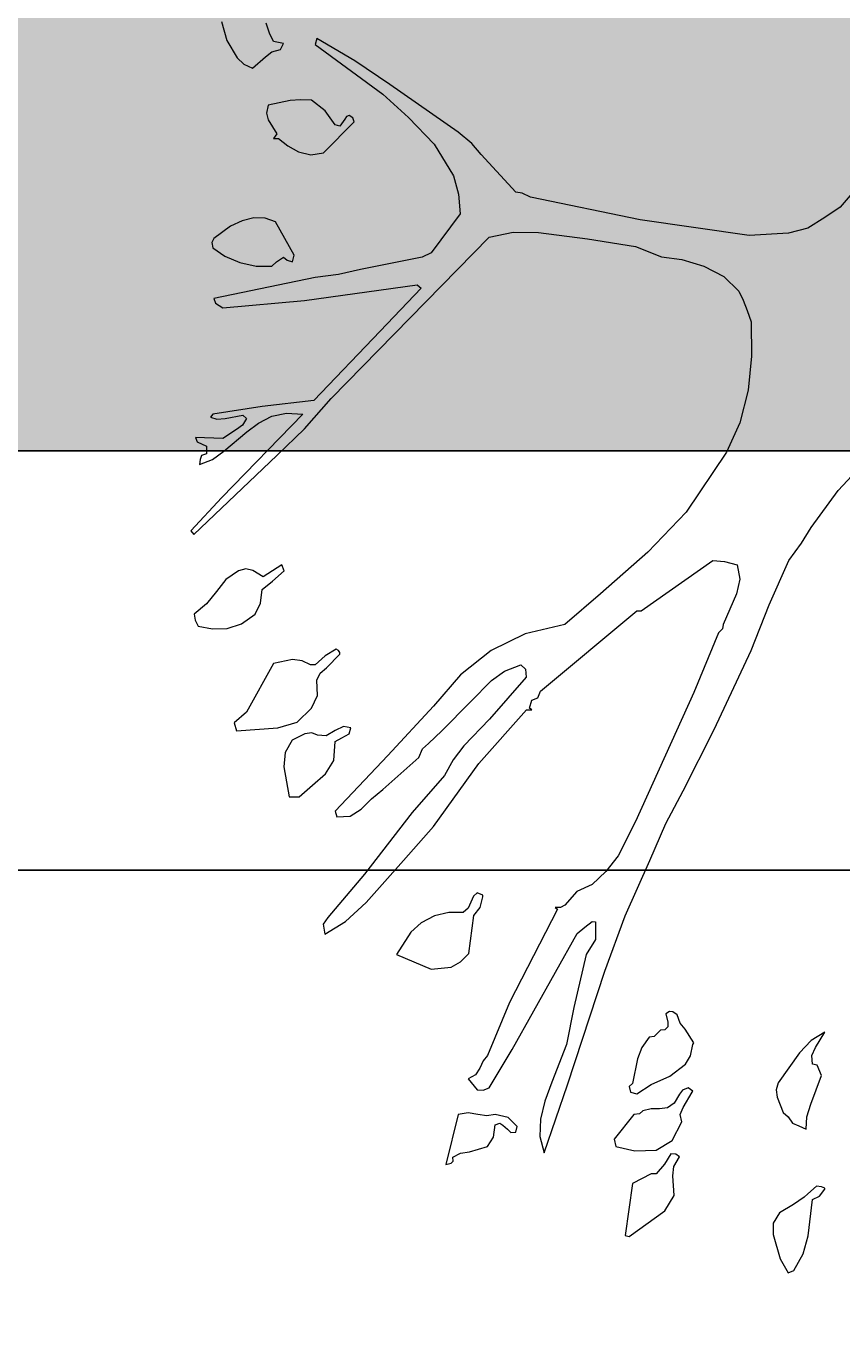
# Model space of a CAD drawing. Units: inches. Extents: x 84 to 1044, y -280 to 906.
# Tile 6 of 105: x 481 to 498, y -132 to -104. Entities that reach past the tile are written whole.
import ezdxf

# ---------------------------------------------------------------- set-up
doc = ezdxf.new("R2010")
doc.units = ezdxf.units.IN
for name, color, linetype, lineweight in [('A-ANNO-DIMS', 2, 'Continuous', 18), ('C-PROP', 7, 'Continuous', 25), ('L-PLNT', 114, 'Continuous', 15)]:
    doc.layers.add(name, color=color, linetype=linetype, lineweight=lineweight)
doc.layers.add('L-PLNT-PATT', color=9, linetype='Continuous', lineweight=9, true_color=0xafd9aa)
doc.styles.get("Standard").update_dxf_attribs({"font": 'arial.ttf'})
doc.dimstyles.get("Standard").update_dxf_attribs({"dimtxt": 0.18, "dimasz": 0.18, "dimexe": 0.18, "dimexo": 0.0625, "dimgap": 0.09, "dimtad": 0, "dimtih": 1, "dimtoh": 1, "dimdec": 4, "dimzin": 0, "dimdsep": 46, "dimtxsty": 'Standard', "dimcen": 0.09, "dimadec": 0, "dimazin": 0, "dimtfac": 1, "dimtdec": 4, "dimtofl": 0, "dimtmove": 0, "dimatfit": 3, "dimfxl": 1, "dimtolj": 1, "dimtzin": 0, "dimarcsym": 0})

# ---------------------------------------------------------------- blocks, each defined once
blk = doc.blocks.new('A$C37E508DF')
for p, q in [((1.3455, 1.0934), (1.3485, 1.102)), ((1.3875, 1.1037), (1.3828, 1.087)), ((1.2713, 1.0694), (1.3044, 1.0887)), ((1.3044, 1.0887), (1.3057, 1.0835)), ((1.3421, 1.0861), (1.3455, 1.0934)), ((1.3057, 1.0835), (1.2469, 1.0402)), ((1.3335, 1.0844), (1.3421, 1.0861)), ((1.3361, 1.0793), (1.3335, 1.0844)), ((1.3434, 1.0771), (1.3361, 1.0793)), ((1.349, 1.0728), (1.3434, 1.0771)), ((1.3828, 1.087), (1.3738, 1.072)), ((1.2409, 1.0488), (1.2713, 1.0694)), ((1.3605, 1.063), (1.349, 1.0728)), ((1.3678, 1.0664), (1.3605, 1.063)), ((1.3738, 1.072), (1.3678, 1.0664)), ((1.1813, 1.0072), (1.2409, 1.0488)), ((1.2469, 1.0402), (1.2246, 1.0201)), ((1.2971, 1.0257), (1.3091, 1.0351)), ((1.3091, 1.0351), (1.3185, 1.0355)), ((1.3185, 1.0355), (1.3275, 1.0347)), ((1.3275, 1.0347), (1.3468, 1.0308)), ((1.2246, 1.0201), (1.2023, 0.9969)), ((1.2718, 1.0162), (1.2731, 1.0197)), ((1.2731, 1.0197), (1.2761, 1.0218)), ((1.2761, 1.0218), (1.2786, 1.0209)), ((1.2786, 1.0209), (1.2799, 1.0184)), ((1.2885, 1.0136), (1.2971, 1.0257)), ((1.3468, 1.0308), (1.3481, 1.0239)), ((1.3481, 1.0239), (1.3468, 1.018)), ((1.2984, 0.9892), (1.2718, 1.0162)), ((1.2799, 1.0184), (1.2842, 1.0124)), ((1.2842, 1.0124), (1.2885, 1.0136)), ((1.3468, 1.018), (1.3391, 1.0059)), ((1.1612, 0.9879), (1.1693, 0.9974)), ((1.1693, 0.9974), (1.1813, 1.0072)), ((1.2023, 0.9969), (1.1852, 0.9691)), ((1.3378, 1.0016), (1.3297, 0.9952)), ((1.3421, 1.0016), (1.3378, 1.0016)), ((1.3391, 1.0059), (1.3421, 1.0016)), ((1.1311, 0.9549), (1.1612, 0.9879)), ((1.3095, 0.9875), (1.2984, 0.9892)), ((1.3202, 0.9901), (1.3095, 0.9875)), ((1.3297, 0.9952), (1.3202, 0.9901)), ((1.1852, 0.9691), (1.1809, 0.9532)), ((0.8383, 0.954), (0.8486, 0.942)), ((1.1183, 0.9506), (1.1256, 0.954)), ((1.1256, 0.954), (1.1311, 0.9549)), ((1.1809, 0.9532), (1.1796, 0.936)), ((0.8486, 0.942), (0.8619, 0.933)), ((1.0227, 0.9309), (1.1183, 0.9506)), ((0.8619, 0.933), (0.8769, 0.9236)), ((0.9279, 0.9172), (1.0227, 0.9309)), ((1.1796, 0.936), (1.2049, 0.9022)), ((1.3241, 0.9), (1.3404, 0.9292)), ((1.3404, 0.9292), (1.3494, 0.9322)), ((1.3494, 0.9322), (1.3592, 0.9326)), ((1.3592, 0.9326), (1.3695, 0.93)), ((1.3695, 0.93), (1.3794, 0.9253)), ((0.8769, 0.9236), (0.8936, 0.9193)), ((0.8936, 0.9193), (0.9279, 0.9172)), ((1.1114, 0.9198), (1.0685, 0.9142)), ((1.1333, 0.9202), (1.1114, 0.9198)), ((1.1543, 0.9159), (1.1333, 0.9202)), ((1.3794, 0.9253), (1.394, 0.9146)), ((1.0269, 0.9077), (1.0042, 0.8987)), ((1.0685, 0.9142), (1.0269, 0.9077)), ((1.2371, 0.8314), (1.1543, 0.9159)), ((1.3948, 0.9065), (1.3846, 0.8992)), ((1.394, 0.9146), (1.3957, 0.9112)), ((1.3957, 0.9112), (1.3948, 0.9065)), ((0.9866, 0.8962), (0.9673, 0.8906)), ((1.0042, 0.8987), (0.9866, 0.8962)), ((1.2049, 0.9022), (1.2126, 0.8983)), ((1.2126, 0.8983), (1.2662, 0.8876)), ((1.3254, 0.8944), (1.3241, 0.9)), ((1.3301, 0.8957), (1.3254, 0.8944)), ((1.3335, 0.8983), (1.3301, 0.8957)), ((1.3395, 0.8944), (1.3335, 0.8983)), ((1.3434, 0.8906), (1.3395, 0.8944)), ((1.3713, 0.8936), (1.3571, 0.8906)), ((1.3846, 0.8992), (1.3713, 0.8936)), ((0.9673, 0.8906), (0.9498, 0.8816)), ((1.2662, 0.8876), (1.2855, 0.8833)), ((1.2855, 0.8833), (1.3057, 0.8807)), ((1.3571, 0.8906), (1.3434, 0.8906)), ((0.9498, 0.8816), (0.9369, 0.8687)), ((1.2169, 0.8743), (1.2135, 0.8713)), ((1.2135, 0.8713), (1.2491, 0.834)), ((1.3151, 0.8606), (1.2169, 0.8743)), ((1.3057, 0.8807), (1.394, 0.8623)), ((0.933, 0.861), (0.9296, 0.852)), ((0.9369, 0.8687), (0.933, 0.861)), ((1.3863, 0.8541), (1.3151, 0.8606)), ((1.394, 0.8623), (1.3927, 0.8584)), ((0.9296, 0.852), (0.9262, 0.8421)), ((1.3927, 0.8584), (1.3863, 0.8541)), ((0.9262, 0.8421), (0.9257, 0.8121)), ((1.2919, 0.7752), (1.2371, 0.8314)), ((1.2491, 0.834), (1.3069, 0.7735)), ((0.9257, 0.8121), (0.9287, 0.7825)), ((0.9287, 0.7825), (0.936, 0.7542)), ((1.3151, 0.7487), (1.2919, 0.7752)), ((1.3069, 0.7735), (1.352, 0.7684)), ((1.352, 0.7684), (1.3948, 0.7615)), ((1.3309, 0.7624), (1.3164, 0.7615)), ((1.3164, 0.7615), (1.3871, 0.6891)), ((1.3434, 0.7598), (1.3309, 0.7624)), ((1.355, 0.7538), (1.3434, 0.7598)), ((1.3687, 0.7607), (1.3657, 0.7577)), ((1.3657, 0.7577), (1.3691, 0.7521)), ((1.3841, 0.7577), (1.3687, 0.7607)), ((1.3914, 0.7572), (1.3841, 0.7577)), ((1.397, 0.759), (1.3914, 0.7572)), ((1.3948, 0.7615), (1.397, 0.759)), ((0.936, 0.7542), (0.9476, 0.7285)), ((1.3391, 0.7255), (1.3151, 0.7487)), ((1.3653, 0.7461), (1.355, 0.7538)), ((1.3854, 0.7294), (1.3653, 0.7461)), ((1.3691, 0.7521), (1.3743, 0.7482)), ((1.3743, 0.7482), (1.3863, 0.7405)), ((1.3863, 0.7405), (1.4099, 0.7414)), ((1.4086, 0.7375), (1.4004, 0.7337)), ((1.4004, 0.7337), (1.4004, 0.7272)), ((1.4099, 0.7414), (1.4086, 0.7375)), ((0.9476, 0.7285), (0.9828, 0.6762)), ((1.4116, 0.6569), (1.3391, 0.7255)), ((1.3953, 0.7221), (1.3854, 0.7294)), ((1.4064, 0.7178), (1.3953, 0.7221)), ((1.4004, 0.7272), (1.4047, 0.7255)), ((1.4047, 0.7255), (1.406, 0.7221)), ((1.406, 0.7221), (1.4064, 0.7178)), ((0.8503, 0.6951), (0.8344, 0.7122)), ((0.8739, 0.6629), (0.8503, 0.6951)), ((1.3871, 0.6891), (1.4141, 0.6599)), ((0.9828, 0.6762), (1.0162, 0.6415)), ((0.8824, 0.6492), (0.8739, 0.6629)), ((1.4141, 0.6599), (1.4116, 0.6569)), ((0.8932, 0.6342), (0.8824, 0.6492)), ((0.9103, 0.5956), (0.8932, 0.6342)), ((0.9382, 0.6303), (0.936, 0.6179)), ((0.9493, 0.6333), (0.9382, 0.6303)), ((0.9596, 0.6342), (0.9493, 0.6333)), ((1.0218, 0.5904), (0.9596, 0.6342)), ((1.0162, 0.6415), (1.0574, 0.605)), ((1.3327, 0.6252), (1.3348, 0.6303)), ((1.3348, 0.6303), (1.3511, 0.62)), ((1.343, 0.6162), (1.3327, 0.6252)), ((1.3511, 0.62), (1.3601, 0.6256)), ((1.3601, 0.6256), (1.3661, 0.6269)), ((1.3661, 0.6269), (1.3725, 0.6252)), ((1.3725, 0.6252), (1.3837, 0.6175)), ((0.936, 0.6179), (0.939, 0.605)), ((1.352, 0.6089), (1.343, 0.6162)), ((1.3533, 0.5969), (1.352, 0.6089)), ((1.3837, 0.6175), (1.3918, 0.6072)), ((0.939, 0.605), (0.9506, 0.5784)), ((1.0574, 0.605), (1.0883, 0.5784)), ((1.358, 0.5874), (1.3533, 0.5969)), ((1.3918, 0.6072), (1.4004, 0.5964)), ((1.4004, 0.5964), (1.4111, 0.5874)), ((0.9262, 0.5557), (0.9103, 0.5956)), ((1.0256, 0.5904), (1.0218, 0.5904)), ((1.1097, 0.5205), (1.0256, 0.5904)), ((1.37, 0.5789), (1.358, 0.5874)), ((1.4111, 0.5874), (1.4103, 0.5823)), ((0.9506, 0.5784), (0.951, 0.5746)), ((0.951, 0.5746), (0.9545, 0.5711)), ((1.0883, 0.5784), (1.123, 0.5703)), ((1.3824, 0.575), (1.37, 0.5789)), ((1.3953, 0.5746), (1.3824, 0.575)), ((1.4077, 0.5771), (1.3953, 0.5746)), ((1.4103, 0.5823), (1.4077, 0.5771)), ((0.9545, 0.5711), (0.9759, 0.5193)), ((1.123, 0.5703), (1.1526, 0.5557)), ((0.9583, 0.4871), (0.9262, 0.5557)), ((1.1526, 0.5557), (1.1792, 0.5347)), ((1.2842, 0.554), (1.2855, 0.5557)), ((1.2842, 0.5527), (1.2842, 0.554)), ((1.2958, 0.5407), (1.2842, 0.5527)), ((1.2855, 0.5557), (1.2876, 0.557)), ((1.2876, 0.557), (1.2971, 0.551)), ((1.2971, 0.551), (1.3057, 0.5433)), ((1.1226, 0.5394), (1.1221, 0.5325)), ((1.1268, 0.5433), (1.1226, 0.5394)), ((1.141, 0.5377), (1.1268, 0.5433)), ((1.3014, 0.536), (1.2958, 0.5407)), ((1.3057, 0.5433), (1.3099, 0.5433)), ((1.3099, 0.5433), (1.3172, 0.5467)), ((1.3172, 0.5467), (1.3254, 0.548)), ((1.3254, 0.548), (1.3421, 0.5446)), ((1.3421, 0.5446), (1.3657, 0.5021)), ((1.1221, 0.5325), (1.1539, 0.4961)), ((1.1521, 0.5296), (1.141, 0.5377)), ((1.1706, 0.5111), (1.1521, 0.5296)), ((1.1792, 0.5347), (1.2027, 0.5072)), ((1.3044, 0.53), (1.3014, 0.536)), ((1.3039, 0.5167), (1.3044, 0.53)), ((0.9759, 0.5193), (1.0269, 0.4069)), ((1.1118, 0.5145), (1.1097, 0.5205)), ((1.3091, 0.5055), (1.3039, 0.5167)), ((1.117, 0.5124), (1.1118, 0.5145)), ((1.1191, 0.5055), (1.117, 0.5124)), ((1.117, 0.5042), (1.1191, 0.5055)), ((1.1217, 0.5042), (1.117, 0.5042)), ((1.1633, 0.4575), (1.1217, 0.5042)), ((1.1955, 0.4858), (1.1706, 0.5111)), ((1.2027, 0.5072), (1.2426, 0.4644)), ((1.3215, 0.4935), (1.3091, 0.5055)), ((1.1539, 0.4961), (1.1762, 0.4729)), ((1.3382, 0.4884), (1.3215, 0.4935)), ((1.3657, 0.5021), (1.3764, 0.4927)), ((1.3764, 0.4927), (1.3743, 0.4858)), ((0.9853, 0.4335), (0.9583, 0.4871)), ((1.207, 0.4747), (1.1955, 0.4858)), ((1.2748, 0.4884), (1.2812, 0.4897)), ((1.2761, 0.4832), (1.2748, 0.4884)), ((1.2825, 0.4798), (1.2761, 0.4832)), ((1.2812, 0.4897), (1.2885, 0.4862)), ((1.2885, 0.4862), (1.2962, 0.4815)), ((1.2962, 0.4815), (1.3039, 0.482)), ((1.3039, 0.482), (1.3087, 0.4841)), ((1.3087, 0.4841), (1.3147, 0.4832)), ((1.3147, 0.4832), (1.3258, 0.4777)), ((1.3743, 0.4858), (1.3382, 0.4884)), ((1.1762, 0.4729), (1.1856, 0.4605)), ((1.2122, 0.47), (1.207, 0.4747)), ((1.2156, 0.4627), (1.2122, 0.47)), ((1.2885, 0.4764), (1.2825, 0.4798)), ((1.2894, 0.4601), (1.2885, 0.4764)), ((1.3258, 0.4777), (1.3318, 0.4669)), ((1.1856, 0.4605), (1.1933, 0.4468)), ((1.2469, 0.4348), (1.2156, 0.4627)), ((1.2426, 0.4644), (1.2885, 0.4159)), ((1.2967, 0.4485), (1.2894, 0.4601)), ((1.3318, 0.4669), (1.3331, 0.4545)), ((1.2027, 0.4026), (1.1633, 0.4575)), ((1.1933, 0.4468), (1.2212, 0.4146)), ((1.3082, 0.4386), (1.2967, 0.4485)), ((1.3331, 0.4545), (1.3284, 0.4284)), ((1.3198, 0.4284), (1.3082, 0.4386)), ((1.0003, 0.4052), (0.9853, 0.4335)), ((1.2568, 0.4266), (1.2469, 0.4348)), ((1.2658, 0.4176), (1.2568, 0.4266)), ((1.3284, 0.4284), (1.3198, 0.4284)), ((1.2212, 0.4146), (1.2628, 0.361)), ((1.2752, 0.4116), (1.2658, 0.4176)), ((1.2885, 0.4159), (1.2868, 0.4108)), ((1.0145, 0.373), (1.0003, 0.4052)), ((1.0269, 0.4069), (1.0419, 0.3769)), ((1.2289, 0.373), (1.2027, 0.4026)), ((1.2868, 0.4108), (1.2752, 0.4116)), ((1.0359, 0.3246), (1.0145, 0.373)), ((1.0419, 0.3769), (1.0527, 0.3632)), ((1.2615, 0.3362), (1.2289, 0.373)), ((1.0527, 0.3632), (1.0647, 0.352)), ((1.2628, 0.361), (1.2949, 0.3233)), ((1.0647, 0.352), (1.078, 0.346)), ((1.078, 0.346), (1.0883, 0.334)), ((1.1599, 0.3426), (1.1646, 0.3447)), ((1.1646, 0.3447), (1.168, 0.3417)), ((1.0883, 0.334), (1.0921, 0.3319)), ((1.1599, 0.3413), (1.1599, 0.3426)), ((1.162, 0.3319), (1.1599, 0.3413)), ((1.168, 0.3417), (1.1702, 0.3366)), ((1.1702, 0.3366), (1.1727, 0.3314)), ((1.2795, 0.3199), (1.2615, 0.3362)), ((1.0535, 0.2766), (1.0359, 0.3246)), ((1.0921, 0.3319), (1.0968, 0.3319)), ((1.0968, 0.3319), (1.0947, 0.3306)), ((1.0947, 0.3306), (1.1367, 0.2491)), ((1.1676, 0.325), (1.162, 0.3319)), ((1.1719, 0.292), (1.1676, 0.325)), ((1.1727, 0.3314), (1.177, 0.3276)), ((1.177, 0.3276), (1.1895, 0.3276)), ((1.1895, 0.3276), (1.2019, 0.3246)), ((1.2019, 0.3246), (1.2135, 0.3186)), ((1.2949, 0.3233), (1.2988, 0.3173)), ((1.0647, 0.3199), (1.0617, 0.3194)), ((1.0617, 0.3194), (1.0617, 0.304)), ((1.0711, 0.3147), (1.0647, 0.3199)), ((1.0775, 0.3092), (1.0711, 0.3147)), ((1.2135, 0.3186), (1.2225, 0.3104)), ((1.2225, 0.3104), (1.2349, 0.2911)), ((1.2975, 0.3087), (1.2795, 0.3199)), ((1.2988, 0.3173), (1.2975, 0.3087)), ((1.0617, 0.304), (1.0698, 0.2911)), ((1.1341, 0.2084), (1.0775, 0.3092)), ((1.0698, 0.2911), (1.0805, 0.2448)), ((1.1792, 0.2847), (1.1719, 0.292)), ((1.2349, 0.2911), (1.2049, 0.2783)), ((1.0861, 0.1775), (1.0535, 0.2766)), ((1.1873, 0.28), (1.1792, 0.2847)), ((1.2049, 0.2783), (1.1873, 0.28)), ((0.9905, 0.2384), (0.9943, 0.241)), ((0.9943, 0.241), (0.9973, 0.2414)), ((0.9973, 0.2414), (1.0003, 0.2393)), ((1.0805, 0.2448), (1.087, 0.2127)), ((1.1367, 0.2491), (1.1556, 0.2032)), ((0.9836, 0.226), (0.9879, 0.2311)), ((0.9879, 0.2311), (0.9905, 0.2384)), ((1.0003, 0.2393), (0.9986, 0.232)), ((0.9986, 0.232), (0.9986, 0.2281)), ((0.8619, 0.2234), (0.8739, 0.2161)), ((0.87, 0.2101), (0.8619, 0.2234)), ((0.9759, 0.214), (0.9836, 0.226)), ((0.9986, 0.2281), (1.0012, 0.2255)), ((1.0012, 0.2255), (1.0051, 0.2251)), ((1.0051, 0.2251), (1.0076, 0.2225)), ((1.0076, 0.2225), (1.0106, 0.2195)), ((1.0106, 0.2195), (1.0149, 0.2191)), ((1.0149, 0.2191), (1.0214, 0.2101)), ((0.8734, 0.2032), (0.87, 0.2101)), ((0.8739, 0.2161), (0.8841, 0.2054)), ((0.9768, 0.2127), (0.9759, 0.214)), ((0.9789, 0.2028), (0.9768, 0.2127)), ((1.0214, 0.2101), (1.0252, 0.2002)), ((1.087, 0.2127), (1.0998, 0.1797)), ((1.1543, 0.1749), (1.1341, 0.2084)), ((0.8687, 0.1947), (0.8726, 0.1955)), ((0.8726, 0.1955), (0.8734, 0.2032)), ((0.8841, 0.2054), (0.9026, 0.1792)), ((0.9832, 0.1955), (0.9789, 0.2028)), ((0.9969, 0.1852), (0.9832, 0.1955)), ((1.0252, 0.2002), (1.0295, 0.1788)), ((1.1556, 0.2032), (1.1594, 0.1985)), ((1.1594, 0.1985), (1.1624, 0.1921)), ((0.8649, 0.1857), (0.8687, 0.1947)), ((0.8743, 0.1608), (0.8649, 0.1857)), ((1.0132, 0.1779), (0.9969, 0.1852)), ((1.1624, 0.1921), (1.1663, 0.1861)), ((1.1663, 0.1861), (1.1727, 0.1827)), ((0.9026, 0.1792), (0.9043, 0.1732)), ((0.9043, 0.1732), (0.9035, 0.1668)), ((0.9768, 0.1719), (0.9811, 0.1749)), ((0.9776, 0.1711), (0.9768, 0.1719)), ((0.9811, 0.1749), (0.9858, 0.1728)), ((0.9858, 0.1728), (0.9884, 0.1694)), ((1.0256, 0.1698), (1.0132, 0.1779)), ((1.0295, 0.1788), (1.0325, 0.1762)), ((1.0325, 0.1762), (1.0312, 0.1711)), ((1.1063, 0.1183), (1.0861, 0.1775)), ((1.0998, 0.1797), (1.1058, 0.1634)), ((1.1594, 0.1728), (1.1543, 0.1749)), ((1.1646, 0.1732), (1.1594, 0.1728)), ((1.1727, 0.1827), (1.1646, 0.1732)), ((0.8777, 0.1496), (0.8743, 0.1608)), ((0.9035, 0.1668), (0.8983, 0.1535)), ((0.9853, 0.1578), (0.9776, 0.1711)), ((0.9884, 0.1694), (0.9931, 0.1616)), ((0.9931, 0.1616), (0.9991, 0.1574)), ((1.0312, 0.1711), (1.0256, 0.1698)), ((1.1058, 0.1634), (1.1097, 0.1475)), ((0.8781, 0.1389), (0.8777, 0.1496)), ((0.894, 0.1496), (0.8902, 0.1441)), ((0.8983, 0.1535), (0.894, 0.1496)), ((0.9879, 0.1518), (0.9853, 0.1578)), ((0.9866, 0.1453), (0.9879, 0.1518)), ((0.9991, 0.1574), (1.0059, 0.1565)), ((1.0059, 0.1565), (1.0132, 0.1565)), ((1.0132, 0.1565), (1.0205, 0.1548)), ((1.0205, 0.1548), (1.0235, 0.1522)), ((1.0235, 0.1522), (1.0282, 0.1518)), ((1.0282, 0.1518), (1.0454, 0.1303)), ((1.1298, 0.1411), (1.1376, 0.1492)), ((1.1376, 0.1492), (1.1491, 0.1518)), ((1.1491, 0.1518), (1.1564, 0.1505)), ((1.1564, 0.1505), (1.1642, 0.1518)), ((1.1642, 0.1518), (1.1727, 0.1531)), ((1.1727, 0.1531), (1.1813, 0.1518)), ((1.1813, 0.1518), (1.192, 0.108)), ((0.8846, 0.1419), (0.8781, 0.1389)), ((0.8902, 0.1441), (0.8846, 0.1419)), ((0.9948, 0.1291), (0.9866, 0.1453)), ((1.1097, 0.1475), (1.1101, 0.1325)), ((1.1311, 0.1364), (1.1298, 0.1411)), ((1.1384, 0.1389), (1.1354, 0.1359)), ((1.1423, 0.1423), (1.1384, 0.1389)), ((1.1449, 0.1441), (1.1423, 0.1423)), ((1.1491, 0.1428), (1.1449, 0.1441)), ((1.1504, 0.132), (1.1491, 0.1428)), ((1.0089, 0.1205), (0.9948, 0.1291)), ((1.0454, 0.1303), (1.0441, 0.1239)), ((1.1101, 0.1325), (1.1063, 0.1183)), ((1.1354, 0.1359), (1.1311, 0.1364)), ((1.1556, 0.1239), (1.1504, 0.132)), ((0.9884, 0.1149), (0.9918, 0.117)), ((0.9935, 0.1063), (0.9884, 0.1149)), ((0.9918, 0.117), (0.9961, 0.1175)), ((0.9961, 0.1175), (1.0016, 0.1085)), ((1.0274, 0.12), (1.0089, 0.1205)), ((1.0441, 0.1239), (1.0274, 0.12)), ((1.1714, 0.1192), (1.1556, 0.1239)), ((1.1792, 0.1179), (1.1714, 0.1192)), ((1.186, 0.1145), (1.1792, 0.1179)), ((0.9943, 0.0982), (0.9935, 0.1063)), ((1.0016, 0.1085), (1.0089, 0.0999)), ((1.1856, 0.111), (1.186, 0.1145)), ((1.1873, 0.1093), (1.1856, 0.111)), ((1.192, 0.108), (1.1873, 0.1093)), ((0.9931, 0.081), (0.9943, 0.0982)), ((1.0089, 0.0999), (1.0132, 0.0999)), ((1.0132, 0.0999), (1.0295, 0.0917)), ((1.0295, 0.0917), (1.0359, 0.0463)), ((0.8619, 0.0875), (0.8649, 0.0887)), ((0.8619, 0.0866), (0.8619, 0.0875)), ((0.8666, 0.0806), (0.8619, 0.0866)), ((0.8649, 0.0887), (0.8691, 0.0892)), ((0.8726, 0.0776), (0.8666, 0.0806)), ((0.8691, 0.0892), (0.8769, 0.0827)), ((0.8769, 0.0827), (0.8799, 0.0797)), ((1.0012, 0.0677), (0.9931, 0.081)), ((0.8764, 0.0459), (0.8726, 0.0776)), ((0.8799, 0.0797), (0.8893, 0.0733)), ((0.8893, 0.0733), (0.9013, 0.066)), ((0.9013, 0.066), (0.9069, 0.057)), ((1.0325, 0.0454), (1.0012, 0.0677)), ((0.8807, 0.0304), (0.8764, 0.0459)), ((0.9069, 0.0471), (0.9009, 0.0261)), ((0.9069, 0.057), (0.9069, 0.0471)), ((1.0359, 0.0463), (1.0325, 0.0454)), ((0.8889, 0.0159), (0.8807, 0.0304)), ((0.9009, 0.0261), (0.894, 0.0137)), ((0.894, 0.0137), (0.8889, 0.0159))]:
    blk.add_line(p, q)
blk = doc.blocks.new('*D60')
at = {"layer": 'A-ANNO-DIMS', "color": 0, "lineweight": -2, "transparency": 16777216}
for p, q in [((134.179, -121.942), (134.179, -180.64)), ((992.074, -121.942), (992.074, -180.64)), ((134.359, -180.46), (562.733, -180.46)), ((991.894, -180.46), (563.521, -180.46))]:
    blk.add_line(p, q, dxfattribs=at)
at = {"layer": 'A-ANNO-DIMS', "color": 0, "transparency": 16777216}
for points in [[(134.359, -180.43), (134.359, -180.49), (134.179, -180.46)], [(991.894, -180.43), (991.894, -180.49), (992.074, -180.46)]]:
    blk.add_solid(points, dxfattribs=at)
at = {"layer": 'Defpoints', "color": 0, "transparency": 16777216}
for p in [(134.179, -121.88), (992.074, -121.88), (992.074, -180.46)]:
    blk.add_point(p, dxfattribs=at)
at = {"layer": 'A-ANNO-DIMS', "color": 0, "transparency": 16777216, "insert": (563.127, -180.46), "char_height": 0.18, "attachment_point": 5}
blk.add_mtext('\\A1;857.9', dxfattribs=at)

msp = doc.modelspace()

# ---------------------------------------------------------------- hatches: boundary and pattern name
at = {"layer": 'L-PLNT-PATT', "transparency": 33554597}
h = msp.add_hatch(color=256, dxfattribs=at)
h.dxf.hatch_style = 1
h.paths.add_polyline_path([(504.574, -40.88), (455.074, -40.88), (455.074, -112.88), (504.574, -112.88)])

# ---------------------------------------------------------------- linework, layer by layer
at = {"layer": 'C-PROP'}
for points in [[(504.574, -112.88), (455.074, -112.88)], [(504.574, -121.88), (455.074, -121.88)]]:
    msp.add_lwpolyline(points, dxfattribs=at)

# ---------------------------------------------------------------- block references
at = {"layer": 'L-PLNT', "xscale": -24.64361536662419, "yscale": 24.64361536662419, "zscale": 24.64361536662419}
msp.add_blockref('A$C37E508DF', (519.355, -130.86), dxfattribs=at)

# ---------------------------------------------------------------- dimensions: what is measured, and where the dimension line sits
at = {"layer": 'A-ANNO-DIMS'}
dim = msp.add_linear_dim(base=(992.074, -180.46), p1=(134.179, -121.88), p2=(992.074, -121.88), dimstyle='Standard', override={"dimdec": 1, "dimlfac": 1, "dimrnd": 0, "dimzin": 0, "dimdsep": 46, "dimlunit": 2}, dxfattribs=at)
dim.commit()
dim.dimension.update_dxf_attribs({"geometry": '*D60', "text_midpoint": (563.127, -180.46)})

doc.saveas('drawing.dxf')
